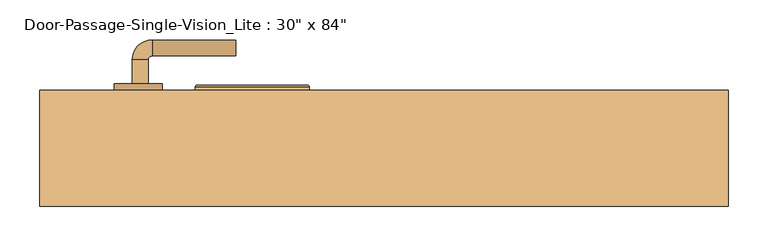
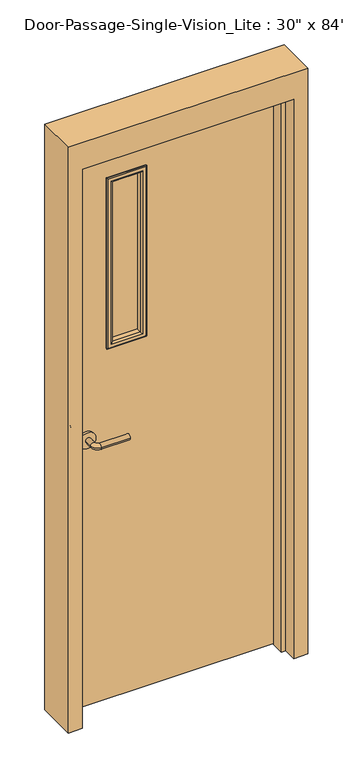
"""IFC4 building model written with IfcOpenShell, lengths in millimetres: door geometry."""

from ifc_helpers import new_model, si_unit, point, frame, frame_2d, origin, place, context, project, spatial, polyline, circle_curve, ellipse_curve, trimmed, segment, composite_curve, outline, extrude, faceted_brep, source, transform, mapped, element, save
from ifc_brep_helpers import plane_surface, cylinder_surface, revolved_surface, advanced_brep


def door_2faac2b1(model_context):
    return source(origin(), model_context, "Body", "SolidModel", [
        advanced_brep(
        [(-315.990625, 4.7, 1016.0), (-295.990625, 4.7, 1016.0), (-295.990625, -25.3, 1016.0), (-315.990625, -25.3, 1016.0), (-290.990625, -30.3, 1016.0), (-290.990625, -50.3, 1016.0), (-185.990625, -50.3, 1016.0), (-185.990625, -30.3, 1016.0)],
        [
            (0, 1, circle_curve(frame((-305.990625, 4.7, 1016.0), z_axis=(0.0, 1.0, 0.0), x_axis=(1.0, 0.0, 0.0)), 10.0)),
            (1, 0, circle_curve(frame((-305.990625, 4.7, 1016.0), z_axis=(0.0, 1.0, 0.0), x_axis=(1.0, 0.0, 0.0)), 10.0)),
            (1, 2),
            (2, 3, circle_curve(frame((-305.990625, -25.3, 1016.0), z_axis=(0.0, 1.0, 0.0), x_axis=(1.0, 0.0, 0.0)), 10.0)),
            (3, 0),
            (3, 2, circle_curve(frame((-305.990625, -25.3, 1016.0), z_axis=(0.0, 1.0, 0.0), x_axis=(1.0, 0.0, 0.0)), 10.0)),
            (4, 5, circle_curve(frame((-290.990625, -40.3, 1016.0), z_axis=(-1.0, 0.0, 0.0), x_axis=(0.0, 1.0, 0.0)), 10.0)),
            (5, 3, circle_curve(frame((-290.990625, -25.3, 1016.0), z_axis=(0.0, 0.0, -1.0), x_axis=(-1.0, 0.0, 0.0)), 25.0)),
            (2, 4, circle_curve(frame((-290.990625, -25.3, 1016.0), z_axis=(0.0, 0.0, 1.0), x_axis=(-1.0, 0.0, 0.0)), 5.0)),
            (5, 4, circle_curve(frame((-290.990625, -40.3, 1016.0), z_axis=(-1.0, 0.0, 0.0), x_axis=(0.0, 1.0, 0.0)), 10.0)),
            (6, 7, circle_curve(frame((-185.990625, -40.3, 1016.0), z_axis=(1.0, 0.0, 0.0), x_axis=(0.0, 1.0, 0.0)), 10.0)),
            (7, 6, circle_curve(frame((-185.990625, -40.3, 1016.0), z_axis=(1.0, 0.0, 0.0), x_axis=(0.0, 1.0, 0.0)), 10.0)),
            (4, 7),
            (6, 5),
        ],
        [
            plane_surface(frame((-305.990625, 4.7, 1016.0), z_axis=(0.0, 1.0, 0.0), x_axis=(0.0, 0.0, 1.0))),
            cylinder_surface(frame((-305.990625, 4.7, 1016.0), z_axis=(0.0, 1.0, 0.0), x_axis=(1.0, 0.0, 0.0)), 10.0),
            revolved_surface(trimmed(ellipse_curve(frame((-305.990625, -25.3, 1016.0), z_axis=(0.0, -1.0, 0.0), x_axis=(1.0, 0.0, 0.0)), 10.0, 10.0), [point((-315.990625, -25.3, 1016.0))], [point((-295.990625, -25.3, 1016.0))], True, "CARTESIAN"), (-290.990625, -25.3, 1016.0), (0.0, 0.0, -1.0)),
            revolved_surface(trimmed(ellipse_curve(frame((-305.990625, -25.3, 1016.0), z_axis=(0.0, -1.0, 0.0), x_axis=(1.0, 0.0, 0.0)), 10.0, 10.0), [point((-295.990625, -25.3, 1016.0))], [point((-315.990625, -25.3, 1016.0))], True, "CARTESIAN"), (-290.990625, -25.3, 1016.0), (0.0, 0.0, -1.0)),
            plane_surface(frame((-185.990625, -40.3, 1016.0), z_axis=(1.0, 0.0, 0.0), x_axis=(0.0, 0.0, 1.0))),
            cylinder_surface(frame((-290.990625, -40.3, 1016.0), z_axis=(-1.0, 0.0, 0.0), x_axis=(0.0, 1.0, 0.0)), 10.0),
        ],
        [
            (0, [[1, 2]]),
            (1, [[3, 4, 5, -2]]),
            (1, [[-5, 6, -3, -1]]),
            (2, [[7, 8, -4, 9]]),
            (3, [[10, -9, -6, -8]]),
            (4, [[11, 12]]),
            (5, [[13, -11, 14, -7]]),
            (5, [[-14, -12, -13, -10]]),
        ],
    ),
        extrude(outline(composite_curve([segment(trimmed(circle_curve(frame_2d((1016.0, -308.490625)), 30.0), [point((1016.0, -338.490625))], [point((1016.0, -278.490625))], False, "CARTESIAN"), True, "CONTINUOUS"), segment(trimmed(circle_curve(frame_2d((1016.0, -308.490625)), 30.0), [point((1016.0, -278.490625))], [point((1016.0, -338.490625))], False, "CARTESIAN"), True, "CONTINUOUS")], self_intersect=False)), frame((0.0, 4.7, 0.0), z_axis=(0.0, 1.0, 0.0), x_axis=(0.0, 0.0, 1.0)), (0.0, 0.0, 1.0), 8.0),
        advanced_brep(
        [(-315.990625, 65.15, 1016.0), (-295.990625, 65.15, 1016.0), (-315.990625, 95.15, 1016.0), (-295.990625, 95.15, 1016.0), (-290.990625, 100.15, 1016.0), (-290.990625, 120.15, 1016.0), (-185.990625, 120.15, 1016.0), (-185.990625, 100.15, 1016.0)],
        [
            (0, 1, circle_curve(frame((-305.990625, 65.15, 1016.0), z_axis=(0.0, -1.0, 0.0), x_axis=(1.0, 0.0, 0.0)), 10.0)),
            (1, 0, circle_curve(frame((-305.990625, 65.15, 1016.0), z_axis=(0.0, -1.0, 0.0), x_axis=(1.0, 0.0, 0.0)), 10.0)),
            (0, 2),
            (2, 3, circle_curve(frame((-305.990625, 95.15, 1016.0), z_axis=(0.0, -1.0, 0.0), x_axis=(1.0, 0.0, 0.0)), 10.0)),
            (3, 1),
            (3, 2, circle_curve(frame((-305.990625, 95.15, 1016.0), z_axis=(0.0, -1.0, 0.0), x_axis=(1.0, 0.0, 0.0)), 10.0)),
            (4, 3, circle_curve(frame((-290.990625, 95.15, 1016.0), z_axis=(0.0, 0.0, 1.0), x_axis=(-1.0, 0.0, 0.0)), 5.0)),
            (2, 5, circle_curve(frame((-290.990625, 95.15, 1016.0), z_axis=(0.0, 0.0, -1.0), x_axis=(-1.0, 0.0, 0.0)), 25.0)),
            (5, 4, circle_curve(frame((-290.990625, 110.15, 1016.0), z_axis=(-1.0, 0.0, 0.0), x_axis=(0.0, -1.0, 0.0)), 10.0)),
            (4, 5, circle_curve(frame((-290.990625, 110.15, 1016.0), z_axis=(-1.0, 0.0, 0.0), x_axis=(0.0, -1.0, 0.0)), 10.0)),
            (6, 7, circle_curve(frame((-185.990625, 110.15, 1016.0), z_axis=(1.0, 0.0, 0.0), x_axis=(0.0, -1.0, 0.0)), 10.0)),
            (7, 6, circle_curve(frame((-185.990625, 110.15, 1016.0), z_axis=(1.0, 0.0, 0.0), x_axis=(0.0, -1.0, 0.0)), 10.0)),
            (5, 6),
            (7, 4),
        ],
        [
            plane_surface(frame((-305.990625, 65.15, 1016.0), z_axis=(0.0, -1.0, 0.0), x_axis=(0.0, 0.0, 1.0))),
            cylinder_surface(frame((-305.990625, 65.15, 1016.0), z_axis=(0.0, -1.0, 0.0), x_axis=(1.0, 0.0, 0.0)), 10.0),
            revolved_surface(trimmed(ellipse_curve(frame((-305.990625, 95.15, 1016.0), z_axis=(0.0, -1.0, 0.0), x_axis=(1.0, 0.0, 0.0)), 10.0, 10.0), [point((-315.990625, 95.15, 1016.0))], [point((-295.990625, 95.15, 1016.0))], True, "CARTESIAN"), (-290.990625, 95.15, 1016.0), (0.0, 0.0, -1.0)),
            revolved_surface(trimmed(ellipse_curve(frame((-305.990625, 95.15, 1016.0), z_axis=(0.0, -1.0, 0.0), x_axis=(1.0, 0.0, 0.0)), 10.0, 10.0), [point((-295.990625, 95.15, 1016.0))], [point((-315.990625, 95.15, 1016.0))], True, "CARTESIAN"), (-290.990625, 95.15, 1016.0), (0.0, 0.0, -1.0)),
            plane_surface(frame((-185.990625, 110.15, 1016.0), z_axis=(1.0, 0.0, 0.0), x_axis=(0.0, 0.0, 1.0))),
            cylinder_surface(frame((-290.990625, 110.15, 1016.0), z_axis=(-1.0, 0.0, 0.0), x_axis=(0.0, -1.0, 0.0)), 10.0),
        ],
        [
            (0, [[1, 2]]),
            (1, [[-1, 3, 4, 5]]),
            (1, [[-2, -5, 6, -3]]),
            (2, [[7, -4, 8, 9]]),
            (3, [[-8, -6, -7, 10]]),
            (4, [[11, 12]]),
            (5, [[-9, 13, -12, 14]]),
            (5, [[-10, -14, -11, -13]]),
        ],
    ),
        extrude(outline(composite_curve([segment(trimmed(circle_curve(frame_2d((1016.0, -308.490625)), 30.0), [point((1016.0, -338.490625))], [point((1016.0, -278.490625))], False, "CARTESIAN"), True, "CONTINUOUS"), segment(trimmed(circle_curve(frame_2d((1016.0, -308.490625)), 30.0), [point((1016.0, -278.490625))], [point((1016.0, -338.490625))], False, "CARTESIAN"), True, "CONTINUOUS")], self_intersect=False)), frame((0.0, 57.15, 0.0), z_axis=(0.0, 1.0, 0.0), x_axis=(0.0, 0.0, 1.0)), (0.0, 0.0, 1.0), 8.0),
        faceted_brep([(381.0, 7.9375, 0.0), (381.0, 57.15, 0.0), (431.8, 57.15, 0.0), (431.8, -88.9, 0.0), (381.0, -88.9, 0.0), (381.0, -39.6875, 0.0), (365.125, -39.6875, 0.0), (365.125, 7.9375, 0.0), (381.0, 7.9375, 2133.6), (381.0, 57.15, 2133.6), (-381.0, 57.15, 2133.6), (-381.0, 57.15, 0.0), (-431.8, 57.15, 0.0), (-431.8, 57.15, 2235.2), (431.8, 57.15, 2235.2), (431.8, -88.9, 2235.2), (-431.8, -88.9, 2235.2), (-431.8, -88.9, 0.0), (-381.0, -88.9, 0.0), (-381.0, -88.9, 2133.6), (381.0, -88.9, 2133.6), (381.0, -39.6875, 2133.6), (-381.0, -39.6875, 2133.6), (-381.0, -39.6875, 0.0), (-365.125, -39.6875, 0.0), (-365.125, -39.6875, 2117.725), (365.125, -39.6875, 2117.725), (365.125, 7.9375, 2117.725), (-365.125, 7.9375, 2117.725), (-365.125, 7.9375, 0.0), (-381.0, 7.9375, 0.0), (-381.0, 7.9375, 2133.6)], [[[0, 1, 2, 3, 4, 5, 6, 7]], [[1, 0, 8, 9]], [[2, 1, 9, 10, 11, 12, 13, 14]], [[3, 2, 14, 15]], [[4, 3, 15, 16, 17, 18, 19, 20]], [[5, 4, 20, 21]], [[6, 5, 21, 22, 23, 24, 25, 26]], [[7, 6, 26, 27]], [[0, 7, 27, 28, 29, 30, 31, 8]], [[9, 8, 31, 10]], [[20, 19, 22, 21]], [[26, 25, 28, 27]], [[12, 11, 30, 29, 24, 23, 18, 17]], [[11, 10, 31, 30]], [[13, 12, 17, 16]], [[19, 18, 23, 22]], [[25, 24, 29, 28]], [[15, 14, 13, 16]]]),
        extrude(outline(polyline([(2133.6, -381.0), (0.0, -381.0), (0.0, 381.0), (2133.6, 381.0), (2133.6, -381.0)]), holes=[polyline([(1981.2, -228.6), (1981.2, -101.6), (1346.2, -101.6), (1346.2, -228.6), (1981.2, -228.6)])]), frame((0.0, 12.7, 0.0), z_axis=(0.0, 1.0, 0.0), x_axis=(0.0, 0.0, 1.0)), (0.0, 0.0, 1.0), 44.45),
        extrude(outline(polyline([(-101.6, 31.75), (-228.6, 31.75), (-228.6, 38.1), (-101.6, 38.1), (-101.6, 31.75)])), frame((0.0, 0.0, 1346.2), z_axis=(0.0, 0.0, 1.0), x_axis=(1.0, 0.0, 0.0)), (0.0, 0.0, 1.0), 635.0),
        advanced_brep(
        [(-228.6, 31.75, 1346.2), (-228.6, 12.7, 1346.2), (-228.6, 12.7, 1981.2), (-228.6, 31.75, 1981.2), (-216.6, 11.7, 1358.2), (-216.6, 31.75, 1358.2), (-216.6, 31.75, 1969.2), (-216.6, 11.7, 1969.2), (-221.6, 6.7, 1353.2), (-221.6, 6.7, 1974.2), (-236.6, 8.7, 1338.2), (-234.6, 6.7, 1340.2), (-234.6, 6.7, 1987.2), (-236.6, 8.7, 1989.2), (-236.6, 12.7, 1338.2), (-236.6, 12.7, 1989.2), (-101.6, 12.7, 1981.2), (-101.6, 31.75, 1981.2), (-113.6, 31.75, 1969.2), (-113.6, 11.7, 1969.2), (-108.6, 6.7, 1974.2), (-95.6, 6.7, 1987.2), (-93.6, 8.7, 1989.2), (-93.6, 12.7, 1989.2), (-101.6, 12.7, 1346.2), (-101.6, 31.75, 1346.2), (-113.6, 31.75, 1358.2), (-113.6, 11.7, 1358.2), (-108.6, 6.7, 1353.2), (-95.6, 6.7, 1340.2), (-93.6, 8.7, 1338.2), (-93.6, 12.7, 1338.2)],
        [
            (0, 1),
            (1, 2),
            (2, 3),
            (3, 0),
            (4, 5),
            (5, 6),
            (6, 7),
            (7, 4),
            (8, 4, ellipse_curve(frame((-221.6, 11.7, 1353.2), z_axis=(-0.7071067811865475, 0.0, 0.7071067811865475), x_axis=(-0.7071067811865474, 0.0, -0.7071067811865476)), 7.0710678, 5.0)),
            (7, 9, ellipse_curve(frame((-221.6, 11.7, 1974.2), z_axis=(-0.7071067811865475, 0.0, -0.7071067811865475), x_axis=(0.7071067811865474, 0.0, -0.7071067811865476)), 7.0710678, 5.0)),
            (9, 8),
            (10, 11, ellipse_curve(frame((-234.6, 8.7, 1340.2), z_axis=(-0.7071067811865475, 0.0, 0.7071067811865475), x_axis=(-0.7071067811865474, 0.0, -0.7071067811865476)), 2.8284271, 2.0)),
            (11, 12),
            (12, 13, ellipse_curve(frame((-234.6, 8.7, 1987.2), z_axis=(-0.7071067811865475, 0.0, -0.7071067811865475), x_axis=(0.7071067811865474, 0.0, -0.7071067811865476)), 2.8284271, 2.0)),
            (13, 10),
            (14, 10),
            (13, 15),
            (15, 14),
            (2, 16),
            (16, 17),
            (17, 3),
            (6, 18),
            (18, 19),
            (19, 7),
            (19, 20, ellipse_curve(frame((-108.6, 11.7, 1974.2), z_axis=(-0.7071067811865475, 0.0, 0.7071067811865475), x_axis=(-0.7071067811865476, 0.0, -0.7071067811865474)), 7.0710678, 5.0)),
            (20, 9),
            (12, 21),
            (21, 22, ellipse_curve(frame((-95.6, 8.7, 1987.2), z_axis=(-0.7071067811865475, 0.0, 0.7071067811865475), x_axis=(-0.7071067811865476, 0.0, -0.7071067811865474)), 2.8284271, 2.0)),
            (22, 13),
            (22, 23),
            (23, 15),
            (16, 24),
            (24, 25),
            (25, 17),
            (18, 26),
            (26, 27),
            (27, 19),
            (27, 28, ellipse_curve(frame((-108.6, 11.7, 1353.2), z_axis=(0.7071067811865475, 0.0, 0.7071067811865475), x_axis=(-0.7071067811865474, 0.0, 0.7071067811865476)), 7.0710678, 5.0)),
            (28, 20),
            (21, 29),
            (29, 30, ellipse_curve(frame((-95.6, 8.7, 1340.2), z_axis=(0.7071067811865475, 0.0, 0.7071067811865475), x_axis=(-0.7071067811865474, 0.0, 0.7071067811865476)), 2.8284271, 2.0)),
            (30, 22),
            (30, 31),
            (31, 23),
            (31, 14),
            (1, 24),
            (0, 25),
            (5, 26),
            (4, 27),
            (8, 28),
            (11, 29),
            (10, 30),
        ],
        [
            plane_surface(frame((-228.6, 12.7, 1346.2), z_axis=(-1.0, 0.0, 0.0), x_axis=(0.0, 0.0, 1.0))),
            plane_surface(frame((-216.6, 31.75, 1358.2), z_axis=(1.0, 0.0, 0.0), x_axis=(0.0, 0.0, 1.0))),
            cylinder_surface(frame((-221.6, 11.7, 1346.2), z_axis=(0.0, 0.0, -1.0), x_axis=(-1.0, 0.0, 0.0)), 5.0),
            cylinder_surface(frame((-234.6, 8.7, 1346.2), z_axis=(0.0, 0.0, -1.0), x_axis=(-1.0, 0.0, 0.0)), 2.0),
            plane_surface(frame((-236.6, 8.7, 1338.2), z_axis=(-1.0, 0.0, 0.0), x_axis=(0.0, 0.0, 1.0))),
            plane_surface(frame((-228.6, 12.7, 1981.2), z_axis=(0.0, 0.0, 1.0), x_axis=(1.0, 0.0, 0.0))),
            plane_surface(frame((-216.6, 31.75, 1969.2), z_axis=(0.0, 0.0, -1.0), x_axis=(1.0, 0.0, 0.0))),
            cylinder_surface(frame((-228.6, 11.7, 1974.2), z_axis=(-1.0, 0.0, 0.0), x_axis=(0.0, 0.0, 1.0)), 5.0),
            cylinder_surface(frame((-228.6, 8.7, 1987.2), z_axis=(-1.0, 0.0, 0.0), x_axis=(0.0, 0.0, 1.0)), 2.0),
            plane_surface(frame((-236.6, 8.7, 1989.2), z_axis=(0.0, 0.0, 1.0), x_axis=(1.0, 0.0, 0.0))),
            plane_surface(frame((-101.6, 12.7, 1981.2), z_axis=(1.0, 0.0, 0.0), x_axis=(0.0, 0.0, -1.0))),
            plane_surface(frame((-113.6, 31.75, 1969.2), z_axis=(-1.0, 0.0, 0.0), x_axis=(0.0, 0.0, -1.0))),
            cylinder_surface(frame((-108.6, 11.7, 1981.2), z_axis=(0.0, 0.0, 1.0), x_axis=(1.0, 0.0, 0.0)), 5.0),
            cylinder_surface(frame((-95.6, 8.7, 1981.2), z_axis=(0.0, 0.0, 1.0), x_axis=(1.0, 0.0, 0.0)), 2.0),
            plane_surface(frame((-93.6, 8.7, 1989.2), z_axis=(1.0, 0.0, 0.0), x_axis=(0.0, 0.0, -1.0))),
            plane_surface(frame((-93.6, 12.7, 1338.2), z_axis=(0.0, 1.0, 0.0), x_axis=(-1.0, 0.0, 0.0))),
            plane_surface(frame((-101.6, 12.7, 1346.2), z_axis=(0.0, 0.0, -1.0), x_axis=(-1.0, 0.0, 0.0))),
            plane_surface(frame((-101.6, 31.75, 1346.2), z_axis=(0.0, 1.0, 0.0), x_axis=(-1.0, 0.0, 0.0))),
            plane_surface(frame((-113.6, 31.75, 1358.2), z_axis=(0.0, 0.0, 1.0), x_axis=(-1.0, 0.0, 0.0))),
            cylinder_surface(frame((-101.6, 11.7, 1353.2), z_axis=(1.0, 0.0, 0.0), x_axis=(0.0, 0.0, -1.0)), 5.0),
            plane_surface(frame((-108.6, 6.7, 1353.2), z_axis=(0.0, -1.0, 0.0), x_axis=(-1.0, 0.0, 0.0))),
            cylinder_surface(frame((-101.6, 8.7, 1340.2), z_axis=(1.0, 0.0, 0.0), x_axis=(0.0, 0.0, -1.0)), 2.0),
            plane_surface(frame((-93.6, 8.7, 1338.2), z_axis=(0.0, 0.0, -1.0), x_axis=(-1.0, 0.0, 0.0))),
        ],
        [
            (0, [[1, 2, 3, 4]]),
            (1, [[5, 6, 7, 8]]),
            (2, [[9, -8, 10, 11]]),
            (3, [[12, 13, 14, 15]]),
            (4, [[16, -15, 17, 18]]),
            (5, [[-3, 19, 20, 21]]),
            (6, [[-7, 22, 23, 24]]),
            (7, [[-10, -24, 25, 26]]),
            (8, [[-14, 27, 28, 29]]),
            (9, [[-17, -29, 30, 31]]),
            (10, [[-20, 32, 33, 34]]),
            (11, [[-23, 35, 36, 37]]),
            (12, [[-25, -37, 38, 39]]),
            (13, [[-28, 40, 41, 42]]),
            (14, [[-30, -42, 43, 44]]),
            (15, [[-31, -44, 45, -18], [46, -32, -19, -2]]),
            (16, [[-33, -46, -1, 47]]),
            (17, [[-21, -34, -47, -4], [48, -35, -22, -6]]),
            (18, [[-36, -48, -5, 49]]),
            (19, [[-38, -49, -9, 50]]),
            (20, [[51, -40, -27, -13], [-26, -39, -50, -11]]),
            (21, [[-41, -51, -12, 52]]),
            (22, [[-43, -52, -16, -45]]),
        ],
    ),
        advanced_brep(
        [(-228.6, 38.1, 1981.2), (-228.6, 57.15, 1981.2), (-228.6, 57.15, 1346.2), (-228.6, 38.1, 1346.2), (-216.6, 58.15, 1969.2), (-216.6, 38.1, 1969.2), (-216.6, 38.1, 1358.2), (-216.6, 58.15, 1358.2), (-221.6, 63.15, 1974.2), (-221.6, 63.15, 1353.2), (-236.6, 61.15, 1989.2), (-234.6, 63.15, 1987.2), (-234.6, 63.15, 1340.2), (-236.6, 61.15, 1338.2), (-236.6, 57.15, 1989.2), (-236.6, 57.15, 1338.2), (-101.6, 57.15, 1346.2), (-101.6, 38.1, 1346.2), (-113.6, 38.1, 1358.2), (-113.6, 58.15, 1358.2), (-108.6, 63.15, 1353.2), (-95.6, 63.15, 1340.2), (-93.6, 61.15, 1338.2), (-93.6, 57.15, 1338.2), (-101.6, 57.15, 1981.2), (-101.6, 38.1, 1981.2), (-113.6, 38.1, 1969.2), (-113.6, 58.15, 1969.2), (-108.6, 63.15, 1974.2), (-95.6, 63.15, 1987.2), (-93.6, 61.15, 1989.2), (-93.6, 57.15, 1989.2)],
        [
            (0, 1),
            (1, 2),
            (2, 3),
            (3, 0),
            (4, 5),
            (5, 6),
            (6, 7),
            (7, 4),
            (8, 4, ellipse_curve(frame((-221.6, 58.15, 1974.2), z_axis=(-0.7071067811865475, 0.0, -0.7071067811865475), x_axis=(-0.7071067811865474, 0.0, 0.7071067811865476)), 7.0710678, 5.0)),
            (7, 9, ellipse_curve(frame((-221.6, 58.15, 1353.2), z_axis=(-0.7071067811865475, 0.0, 0.7071067811865475), x_axis=(0.7071067811865474, 0.0, 0.7071067811865476)), 7.0710678, 5.0)),
            (9, 8),
            (10, 11, ellipse_curve(frame((-234.6, 61.15, 1987.2), z_axis=(-0.7071067811865475, 0.0, -0.7071067811865475), x_axis=(-0.7071067811865474, 0.0, 0.7071067811865476)), 2.8284271, 2.0)),
            (11, 12),
            (12, 13, ellipse_curve(frame((-234.6, 61.15, 1340.2), z_axis=(-0.7071067811865475, 0.0, 0.7071067811865475), x_axis=(0.7071067811865474, 0.0, 0.7071067811865476)), 2.8284271, 2.0)),
            (13, 10),
            (14, 10),
            (13, 15),
            (15, 14),
            (2, 16),
            (16, 17),
            (17, 3),
            (6, 18),
            (18, 19),
            (19, 7),
            (19, 20, ellipse_curve(frame((-108.6, 58.15, 1353.2), z_axis=(-0.7071067811865475, 0.0, -0.7071067811865475), x_axis=(-0.7071067811865476, 0.0, 0.7071067811865474)), 7.0710678, 5.0)),
            (20, 9),
            (12, 21),
            (21, 22, ellipse_curve(frame((-95.6, 61.15, 1340.2), z_axis=(-0.7071067811865475, 0.0, -0.7071067811865475), x_axis=(-0.7071067811865476, 0.0, 0.7071067811865474)), 2.8284271, 2.0)),
            (22, 13),
            (22, 23),
            (23, 15),
            (16, 24),
            (24, 25),
            (25, 17),
            (18, 26),
            (26, 27),
            (27, 19),
            (27, 28, ellipse_curve(frame((-108.6, 58.15, 1974.2), z_axis=(0.7071067811865475, 0.0, -0.7071067811865475), x_axis=(-0.7071067811865474, 0.0, -0.7071067811865476)), 7.0710678, 5.0)),
            (28, 20),
            (21, 29),
            (29, 30, ellipse_curve(frame((-95.6, 61.15, 1987.2), z_axis=(0.7071067811865475, 0.0, -0.7071067811865475), x_axis=(-0.7071067811865474, 0.0, -0.7071067811865476)), 2.8284271, 2.0)),
            (30, 22),
            (30, 31),
            (31, 23),
            (31, 14),
            (1, 24),
            (0, 25),
            (5, 26),
            (4, 27),
            (8, 28),
            (11, 29),
            (10, 30),
        ],
        [
            plane_surface(frame((-228.6, 57.15, 1981.2), z_axis=(-1.0, 0.0, 0.0), x_axis=(0.0, 0.0, -1.0))),
            plane_surface(frame((-216.6, 38.1, 1969.2), z_axis=(1.0, 0.0, 0.0), x_axis=(0.0, 0.0, -1.0))),
            cylinder_surface(frame((-221.6, 58.15, 1981.2), z_axis=(0.0, 0.0, 1.0), x_axis=(-1.0, 0.0, 0.0)), 5.0),
            cylinder_surface(frame((-234.6, 61.15, 1981.2), z_axis=(0.0, 0.0, 1.0), x_axis=(-1.0, 0.0, 0.0)), 2.0),
            plane_surface(frame((-236.6, 61.15, 1989.2), z_axis=(-1.0, 0.0, 0.0), x_axis=(0.0, 0.0, -1.0))),
            plane_surface(frame((-228.6, 57.15, 1346.2), z_axis=(0.0, 0.0, -1.0), x_axis=(1.0, 0.0, 0.0))),
            plane_surface(frame((-216.6, 38.1, 1358.2), z_axis=(0.0, 0.0, 1.0), x_axis=(1.0, 0.0, 0.0))),
            cylinder_surface(frame((-228.6, 58.15, 1353.2), z_axis=(-1.0, 0.0, 0.0), x_axis=(0.0, 0.0, -1.0)), 5.0),
            cylinder_surface(frame((-228.6, 61.15, 1340.2), z_axis=(-1.0, 0.0, 0.0), x_axis=(0.0, 0.0, -1.0)), 2.0),
            plane_surface(frame((-236.6, 61.15, 1338.2), z_axis=(0.0, 0.0, -1.0), x_axis=(1.0, 0.0, 0.0))),
            plane_surface(frame((-101.6, 57.15, 1346.2), z_axis=(1.0, 0.0, 0.0), x_axis=(0.0, 0.0, 1.0))),
            plane_surface(frame((-113.6, 38.1, 1358.2), z_axis=(-1.0, 0.0, 0.0), x_axis=(0.0, 0.0, 1.0))),
            cylinder_surface(frame((-108.6, 58.15, 1346.2), z_axis=(0.0, 0.0, -1.0), x_axis=(1.0, 0.0, 0.0)), 5.0),
            cylinder_surface(frame((-95.6, 61.15, 1346.2), z_axis=(0.0, 0.0, -1.0), x_axis=(1.0, 0.0, 0.0)), 2.0),
            plane_surface(frame((-93.6, 61.15, 1338.2), z_axis=(1.0, 0.0, 0.0), x_axis=(0.0, 0.0, 1.0))),
            plane_surface(frame((-93.6, 57.15, 1989.2), z_axis=(0.0, -1.0, 0.0), x_axis=(-1.0, 0.0, 0.0))),
            plane_surface(frame((-101.6, 57.15, 1981.2), z_axis=(0.0, 0.0, 1.0), x_axis=(-1.0, 0.0, 0.0))),
            plane_surface(frame((-101.6, 38.1, 1981.2), z_axis=(0.0, -1.0, 0.0), x_axis=(-1.0, 0.0, 0.0))),
            plane_surface(frame((-113.6, 38.1, 1969.2), z_axis=(0.0, 0.0, -1.0), x_axis=(-1.0, 0.0, 0.0))),
            cylinder_surface(frame((-101.6, 58.15, 1974.2), z_axis=(1.0, 0.0, 0.0), x_axis=(0.0, 0.0, 1.0)), 5.0),
            plane_surface(frame((-108.6, 63.15, 1974.2), z_axis=(0.0, 1.0, 0.0), x_axis=(-1.0, 0.0, 0.0))),
            cylinder_surface(frame((-101.6, 61.15, 1987.2), z_axis=(1.0, 0.0, 0.0), x_axis=(0.0, 0.0, 1.0)), 2.0),
            plane_surface(frame((-93.6, 61.15, 1989.2), z_axis=(0.0, 0.0, 1.0), x_axis=(-1.0, 0.0, 0.0))),
        ],
        [
            (0, [[1, 2, 3, 4]]),
            (1, [[5, 6, 7, 8]]),
            (2, [[9, -8, 10, 11]]),
            (3, [[12, 13, 14, 15]]),
            (4, [[16, -15, 17, 18]]),
            (5, [[-3, 19, 20, 21]]),
            (6, [[-7, 22, 23, 24]]),
            (7, [[-10, -24, 25, 26]]),
            (8, [[-14, 27, 28, 29]]),
            (9, [[-17, -29, 30, 31]]),
            (10, [[-20, 32, 33, 34]]),
            (11, [[-23, 35, 36, 37]]),
            (12, [[-25, -37, 38, 39]]),
            (13, [[-28, 40, 41, 42]]),
            (14, [[-30, -42, 43, 44]]),
            (15, [[-31, -44, 45, -18], [46, -32, -19, -2]]),
            (16, [[-33, -46, -1, 47]]),
            (17, [[-21, -34, -47, -4], [48, -35, -22, -6]]),
            (18, [[-36, -48, -5, 49]]),
            (19, [[-38, -49, -9, 50]]),
            (20, [[51, -40, -27, -13], [-26, -39, -50, -11]]),
            (21, [[-41, -51, -12, 52]]),
            (22, [[-43, -52, -16, -45]]),
        ],
    ),
    ])


if __name__ == "__main__":
    model = new_model("IFC4")
    model_context = context("Model", 3, world=origin())
    ifc_project = project(units=[si_unit("LENGTHUNIT", "METRE", prefix="MILLI")], contexts=[model_context])
    site = spatial("IfcSite", under=ifc_project)
    building = spatial("IfcBuilding", under=site)
    placement = place(None, origin())
    door_shape = door_2faac2b1(model_context)
    element("IfcDoor", 1, ObjectType="Door-Passage-Single-Vision_Lite : 30\" x 84\"", at=placement, inside=building, context=model_context, shape_type="MappedRepresentation", body=[
        mapped(door_shape, transform((0.0, 0.0, 0.0), x_axis=(1.0, 0.0, 0.0), y_axis=(0.0, 1.0, 0.0), z_axis=(0.0, 0.0, 1.0))),
    ])
    save(model, "model.ifc")

# Revit data of these elements
# Type "Door-Passage-Single-Vision_Lite : 30\" x 84\""
#   Type Mark = "20"
#   Assembly Code = "B2030100"
#   Analytic Construction = "Wooden"
#   Thickness = 0' - 1 3/4"
#   Thermal Resistance (R) = 2.5876 (h·ft²·°F)/BTU
#   Swing Angle [instance default] = 90.00°
#   Strike Height = 3' - 4"
#   Rough Width [instance default] = 2' - 10"
#   Rough Height [instance default] = 7' - 4"
#   MFOpeningHeight [instance default] = 0' - 4"
#   MFOpeningWidth [instance default] = 0' - 4"
#   Inset Calculate [instance default] = 0' - 4"
#   Masonry Inset [instance default] = 0' - 1"
#   Height = 7' - 0"
#   Width = 2' - 6"
#   Heat Transfer Coefficient (U) = 0.3865 BTU/(h·ft²·°F)
#   Masonry Frame Depth = 0' - 5 3/4"
#   Masonry Frame [instance default] = yes
#   Function = 1
#   Dry Wall Frame [instance default] = no
#   Define Thermal Properties by = 1
#   Panel Material = Wood - Birch
#   Glazing = Glass
#   Glass Stop Material = Metal - Paint Finish - Grey
#   Frame Material = Metal - Paint Finish - Grey
#   Door Handle Material = Aluminum
#   Visual Light Transmittance = 0
#   Solar Heat Gain Coefficient = 0
#   Wall Closure = (empty or 0)
# Element 1 (IfcDoor, "Door-Passage-Single-Vision_Lite : 30\" x 84\"")
#   Materials on its faces: "Metal - Paint Finish - Grey", "Aluminum", "Wood - Birch", "Glass"
# Materials
#   "Wood - Birch": class "Wood", colour RGB 173 132 96, transparency 0, Cost = 0
#   "Glass": class "Glass", colour RGB 245 245 243, transparency 1, Description = "Soda Lime Glass", Cost = 0
#   "Metal - Paint Finish - Grey": class "Paint", colour RGB 178 178 178, transparency 0, Cost = 0
#   "Aluminum": class "Metal", colour RGB 244 245 246, transparency 0, Description = "Aluminum 6061", Cost = 0
